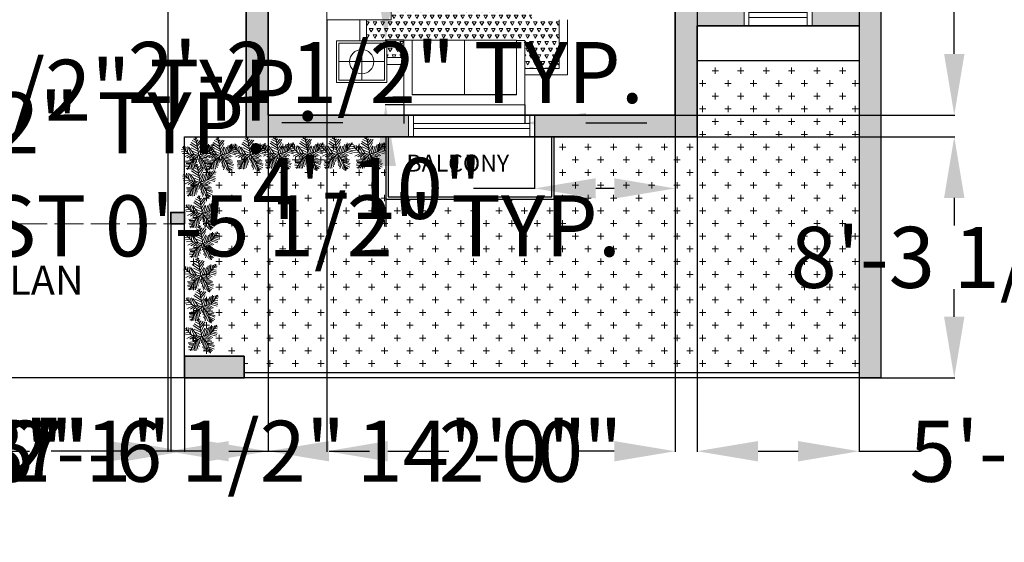
# Model space of a CAD drawing. Units: inches. Extents: x 29 to 6336, y 3 to 2592.
# Tile 4 of 8: x 5531 to 5938, y 1885 to 2100. Entities that reach past the tile are written whole.
import ezdxf

# ---------------------------------------------------------------- set-up
doc = ezdxf.new("R2010")
doc.units = ezdxf.units.IN
doc.header["$MEASUREMENT"] = 0
doc.linetypes.add('ACAD_ISO02W100', pattern=[15, 12, -3])
for name, color, linetype, lineweight in [('A-ANNO-DIMS', 2, 'Continuous', 18), ('A-ANNO-TEXT', 7, 'Continuous', 25), ('A-AREA-IDEN', 7, 'Continuous', 18), ('A-COLS', 7, 'Continuous', 35), ('A-COLS-PATT', 18, 'Continuous', 13), ('A-FLOR', 7, 'Continuous', 25), ('A-FLOR-OVHD', 8, 'ACAD_ISO02W100', 18), ('A-FLOR-PATT', 9, 'Continuous', 13), ('A-FURN', 8, 'Continuous', 18), ('A-GLAZ', 116, 'Continuous', 18), ('A-WALL', 7, 'Continuous', 35), ('A-WALL-PATT', 242, 'Continuous', 13), ('C-PROP', 7, 'Continuous', 25), ('L-PLNT', 94, 'Continuous', 18), ('L-PLNT-PATT', 114, 'Continuous', 13)]:
    doc.layers.add(name, color=color, linetype=linetype, lineweight=lineweight)
doc.styles.get("Standard").update_dxf_attribs({"font": 'arial.ttf'})
doc.dimstyles.get("Standard").update_dxf_attribs({"dimtxt": 25.18, "dimasz": 25.18, "dimexe": 0.18, "dimexo": 0.0625, "dimgap": 0.09, "dimtad": 0, "dimtih": 1, "dimtoh": 1, "dimdec": 0, "dimzin": 0, "dimdsep": 46, "dimlunit": 3, "dimtxsty": 'Standard', "dimcen": 0.09, "dimadec": 0, "dimazin": 0, "dimtfac": 1, "dimtdec": 0, "dimtofl": 0, "dimtmove": 0, "dimatfit": 3, "dimfxl": 1, "dimtolj": 1, "dimtzin": 0, "dimarcsym": 0})

# ---------------------------------------------------------------- blocks, each defined once
blk = doc.blocks.new('*U2')
for p, q in [((-3.665, 19.273), (-27.574, 35.527)), ((-5.114, 28.097), (-24.676, 40.636)), ((-7.288, 39.707), (-21.778, 46.673)), ((-8.737, 47.138), (-17.069, 52.711)), ((-10.186, 53.64), (-13.084, 55.962)), ((0, 0), (-10.5, 57)), ((-9.099, 51.782), (-6.563, 55.962)), ((-7.65, 43.423), (-2.578, 49.46)), ((-5.839, 35.992), (4.667, 48.067)), ((-5.114, 27.632), (10.463, 46.673)), ((-2.941, 16.486), (8.652, 37.85)), ((16.259, 5.805), (23.142, 31.348)), ((22.055, 7.198), (27.489, 32.277)), ((27, 9), (48, 36)), ((27.127, 9.056), (31.112, 35.992)), ((35.096, 32.741), (37.27, 22.524)), ((38.719, 34.134), (41.979, 28.561)), ((44.153, 36.456), (45.239, 32.741)), ((-47.498, 19.737), (-55.83, 18.344)), ((-40.615, 13.7), (-55.105, 10.913)), ((-31.5, 4.5), (-52.5, 25.5)), ((-33.37, 6.269), (-52.207, 5.34)), ((-48.585, 21.131), (-49.309, 29.026)), ((-28.299, 3.483), (-47.86, -5.805)), ((-43.513, 28.561), (-42.427, 15.558)), ((-38.442, 26.239), (-34.819, 7.663)), ((-21.416, 3.018), (-38.079, -8.128)), ((-35.544, 28.097), (-24.314, 3.947)), ((0, 0), (-31.5, 4.5)), ((-14.533, 2.09), (-30.834, 25.31)), ((-15.982, 2.09), (-30.11, -9.521)), ((-24.314, 23.917), (-2.941, 13.7)), ((0, 0), (-22.5, -19.5)), ((-6.563, 1.161), (-21.416, -8.128)), ((-20.691, 13.7), (-1.129, 4.876)), ((-1.129, 6.734), (9.014, 26.704)), ((0, 0), (27, 9)), ((0, 0), (18, -22.5)), ((3.942, 1.625), (11.187, 24.381)), ((6.478, 1.625), (26.04, -8.592)), ((10.101, 3.483), (17.708, 26.239)), ((11.187, 3.483), (30.749, -5.805)), ((18.07, 5.805), (35.096, -3.483)), ((24.229, 7.663), (46.688, 1.625)), ((29.662, 12.307), (48.137, 6.269)), ((31.836, 30.883), (32.561, 16.486)), ((33.285, 16.486), (48.862, 10.913)), ((36.183, 19.737), (48.137, 17.88)), ((40.53, 25.775), (48.862, 24.846)), ((43.791, 29.954), (51.036, 30.883)), ((-17.431, -15.094), (-42.789, -18.809)), ((-28.299, -29.026), (-42.789, -31.348)), ((-24.314, -21.596), (-42.427, -22.06)), ((-26.849, -26.24), (-40.253, -25.775)), ((-22.5, -19.5), (-37.5, -45)), ((-15.257, -12.772), (-30.11, -12.772)), ((-29.023, -30.884), (-27.936, -43.887)), ((-25.038, -23.918), (-22.865, -45.281)), ((-20.691, -18.345), (-17.793, -44.352)), ((-6.563, -5.805), (-19.967, -9.985)), ((-17.069, -15.094), (-12.721, -40.172)), ((-13.446, -11.378), (-8.737, -32.741)), ((-9.461, -8.592), (-6.201, -23.453)), ((-4.752, -3.483), (-3.665, -14.629)), ((2.493, -3.019), (-1.491, -20.202)), ((1.769, -2.555), (24.229, -9.521)), ((5.029, -6.27), (2.131, -25.775)), ((9.014, -11.378), (3.58, -35.992)), ((14.085, -16.951), (6.478, -40.172)), ((7.565, -9.056), (32.198, -14.629)), ((18.07, -22.524), (8.289, -45.745)), ((12.274, -15.094), (36.907, -18.809)), ((20.244, -30.419), (15.897, -44.816)), ((16.259, -19.738), (36.183, -22.989)), ((18, -22.5), (27, -52.5)), ((18.433, -22.524), (40.53, -29.026)), ((19.157, -25.311), (38.719, -33.206)), ((-30.834, -34.135), (-42.427, -35.528)), ((-34.457, -39.708), (-40.978, -42.494)), ((-32.646, -36.921), (-31.921, -44.352)), ((22.78, -37.85), (19.519, -48.532)), ((21.331, -32.741), (39.081, -40.636)), ((22.78, -38.314), (34.372, -44.816)), ((24.591, -45.745), (23.142, -50.854)), ((24.591, -43.423), (30.749, -47.603)), ((26.764, -49.925), (28.213, -50.854))]:
    blk.add_line(p, q)
blk = doc.blocks.new('WIN-48')
for p, q in [((0, 9), (0, 0)), ((2, 9), (2, 0)), ((50, 9), (50, 0)), ((52, 9), (52, 0)), ((2, 5.5), (50, 5.5)), ((2, 3.5), (50, 3.5))]:
    blk.add_line(p, q)
blk = doc.blocks.new('WIN-24')
for p, q in [((0, 9), (0, 0)), ((2, 9), (2, 0)), ((26, 9), (26, 0)), ((28, 9), (28, 0)), ((2, 5.5), (26, 5.5)), ((2, 3.5), (26, 3.5))]:
    blk.add_line(p, q)
blk = doc.blocks.new('SOFA-TWO-SEAT')
blk.add_line((4.12, 24.97), (26.62, 24.97))
for points in [[(4.17, 49.94), (0, 49.94), (0, 0), (4.17, 0)], [(4.17, 49.94), (26.62, 49.94), (26.62, 46.51), (4.17, 46.51)], [(4.17, 3.43), (4.17, 46.51)], [(4.12, 3.43), (26.57, 3.43), (26.57, 0), (4.12, 0)]]:
    blk.add_lwpolyline(points)
blk.add_lwpolyline([(26.62, 46.51), (4.12, 46.51), (4.12, 3.43), (26.62, 3.43)], close=True)
blk = doc.blocks.new('END-TABLE-21X17')
for p, q in [((10.41, 16.21), (10.41, 1)), ((1, 8.6), (19.81, 8.6))]:
    blk.add_line(p, q)
for points in [[(0, 17.21), (20.81, 17.21), (20.81, 0), (0, 0)], [(1, 16.21), (19.81, 16.21), (19.81, 1), (1, 1)]]:
    blk.add_lwpolyline(points, close=True)
blk.add_circle((10.41, 8.6), 5)
blk = doc.blocks.new('PORCH-POST')
blk.add_lwpolyline([(5.63, 0), (0, 0), (0, 4.72), (5.63, 4.72)], close=True)
blk = doc.blocks.new('*D28')
at = {"layer": 'A-ANNO-DIMS', "color": 0, "lineweight": -2, "transparency": 16777216}
for p, q in [((5689.81, 2064.89), (5689.81, 2057.28)), ((5739.75, 2064.89), (5739.75, 2057.28)), ((5664.63, 2057.46), (5639.45, 2057.46)), ((5764.93, 2057.46), (5790.11, 2057.46))]:
    blk.add_line(p, q, dxfattribs=at)
at = {"layer": 'A-ANNO-DIMS', "color": 0, "transparency": 16777216}
for points in [[(5664.63, 2061.65), (5664.63, 2053.26), (5689.81, 2057.46)], [(5764.93, 2061.65), (5764.93, 2053.26), (5739.75, 2057.46)]]:
    blk.add_solid(points, dxfattribs=at)
at = {"layer": 'Defpoints', "color": 0, "transparency": 16777216}
for p in [(5689.81, 2064.95), (5739.75, 2064.95), (5689.81, 2057.46)]:
    blk.add_point(p, dxfattribs=at)
at = {"layer": 'A-ANNO-DIMS', "color": 0, "transparency": 16777216, "insert": (5509.91, 2057.46), "char_height": 25.18, "attachment_point": 5}
blk.add_mtext('\\A1;SOFA 4\'-2" TYP.', dxfattribs=at)
blk = doc.blocks.new('*D29')
at = {"layer": 'A-ANNO-DIMS', "color": 0, "lineweight": -2, "transparency": 16777216}
for p, q in [((5682.32, 2116.75), (5682.32, 2141.93)), ((5689.75, 2091.57), (5682.14, 2091.57)), ((5689.75, 2064.95), (5682.14, 2064.95)), ((5682.32, 2039.77), (5682.32, 2014.59))]:
    blk.add_line(p, q, dxfattribs=at)
at = {"layer": 'A-ANNO-DIMS', "color": 0, "transparency": 16777216}
for points in [[(5678.12, 2116.75), (5686.52, 2116.75), (5682.32, 2091.57)], [(5678.12, 2039.77), (5686.52, 2039.77), (5682.32, 2064.95)]]:
    blk.add_solid(points, dxfattribs=at)
at = {"layer": 'Defpoints', "color": 0, "transparency": 16777216}
for p in [(5682.32, 2091.57), (5689.81, 2091.57), (5689.81, 2064.95)]:
    blk.add_point(p, dxfattribs=at)
at = {"layer": 'A-ANNO-DIMS', "color": 0, "transparency": 16777216, "insert": (5682.32, 2078.26), "char_height": 25.18, "attachment_point": 5}
blk.add_mtext('\\A1;2\'-2 1/2" TYP.', dxfattribs=at)
blk = doc.blocks.new('*D34')
at = {"layer": 'A-ANNO-DIMS', "color": 0, "lineweight": -2, "transparency": 16777216}
for p, q in [((5638.44, 2177.3), (5613.26, 2177.3)), ((5663.62, 2174.24), (5663.62, 2177.48)), ((5684.43, 2174.24), (5684.43, 2177.48)), ((5709.61, 2177.3), (5734.79, 2177.3))]:
    blk.add_line(p, q, dxfattribs=at)
at = {"layer": 'A-ANNO-DIMS', "color": 0, "transparency": 16777216}
for points in [[(5638.44, 2181.49), (5638.44, 2173.1), (5663.62, 2177.3)], [(5709.61, 2181.49), (5709.61, 2173.1), (5684.43, 2177.3)]]:
    blk.add_solid(points, dxfattribs=at)
at = {"layer": 'Defpoints', "color": 0, "transparency": 16777216}
for p in [(5663.62, 2174.18), (5684.43, 2177.3), (5684.43, 2174.18)]:
    blk.add_point(p, dxfattribs=at)
at = {"layer": 'A-ANNO-DIMS', "color": 0, "transparency": 16777216, "insert": (5913.59, 2177.3), "char_height": 25.18, "attachment_point": 5}
blk.add_mtext('\\A1;END TABLE 1\'-9" TYP.', dxfattribs=at)
blk = doc.blocks.new('*D38')
at = {"layer": 'A-ANNO-DIMS', "color": 0, "lineweight": -2, "transparency": 16777216}
for p, q in [((5410.6, 2015.81), (5410.6, 2014.84)), ((5416.23, 2015.81), (5416.23, 2014.84)), ((5385.42, 2015.02), (5360.24, 2015.02)), ((5441.41, 2015.02), (5466.59, 2015.02))]:
    blk.add_line(p, q, dxfattribs=at)
at = {"layer": 'A-ANNO-DIMS', "color": 0, "transparency": 16777216}
for points in [[(5385.42, 2019.22), (5385.42, 2010.83), (5410.6, 2015.02)], [(5441.41, 2019.22), (5441.41, 2010.83), (5416.23, 2015.02)]]:
    blk.add_solid(points, dxfattribs=at)
at = {"layer": 'Defpoints', "color": 0, "transparency": 16777216}
for p in [(5410.6, 2015.87), (5416.23, 2015.87), (5416.23, 2015.02)]:
    blk.add_point(p, dxfattribs=at)
at = {"layer": 'A-ANNO-DIMS', "color": 0, "transparency": 16777216, "insert": (5624.9, 2015.02), "char_height": 25.18, "attachment_point": 5}
blk.add_mtext('\\A1;POST 0\'-5 1/2" TYP.', dxfattribs=at)
blk = doc.blocks.new('*D39')
at = {"layer": 'A-ANNO-DIMS', "color": 0, "lineweight": -2, "transparency": 16777216}
for p, q in [((5417.07, 2045.77), (5417.07, 2070.95)), ((5417.07, 2070.95), (5442.25, 2070.95)), ((5416.29, 2020.59), (5417.25, 2020.59)), ((5416.29, 2015.87), (5417.25, 2015.87)), ((5417.07, 1990.69), (5417.07, 1965.51))]:
    blk.add_line(p, q, dxfattribs=at)
at = {"layer": 'A-ANNO-DIMS', "color": 0, "transparency": 16777216}
for points in [[(5412.88, 2045.77), (5421.27, 2045.77), (5417.07, 2020.59)], [(5412.88, 1990.69), (5421.27, 1990.69), (5417.07, 2015.87)]]:
    blk.add_solid(points, dxfattribs=at)
at = {"layer": 'Defpoints', "color": 0, "transparency": 16777216}
for p in [(5416.23, 2020.59), (5417.07, 2020.59), (5416.23, 2015.87)]:
    blk.add_point(p, dxfattribs=at)
at = {"layer": 'A-ANNO-DIMS', "color": 0, "transparency": 16777216, "insert": (5548.42, 2070.95), "char_height": 25.18, "attachment_point": 5}
blk.add_mtext('\\A1;0\'-4 1/2" TYP.', dxfattribs=at)
blk = doc.blocks.new('*D49')
at = {"layer": 'A-ANNO-DIMS', "color": 0, "lineweight": -2, "transparency": 16777216}
for p, q in [((5419.6, 2191.59), (5419.6, 1921.9)), ((5510.11, 2191.59), (5510.11, 1921.9)), ((5444.78, 1922.08), (5484.93, 1922.08)), ((5510.11, 1922.08), (5535.29, 1922.08))]:
    blk.add_line(p, q, dxfattribs=at)
at = {"layer": 'A-ANNO-DIMS', "color": 0, "transparency": 16777216}
for points in [[(5444.78, 1926.28), (5444.78, 1917.88), (5419.6, 1922.08)], [(5484.93, 1926.28), (5484.93, 1917.88), (5510.11, 1922.08)]]:
    blk.add_solid(points, dxfattribs=at)
at = {"layer": 'Defpoints', "color": 0, "transparency": 16777216}
for p in [(5419.6, 2191.65), (5510.11, 2191.65), (5510.11, 1922.08)]:
    blk.add_point(p, dxfattribs=at)
at = {"layer": 'A-ANNO-DIMS', "color": 0, "transparency": 16777216, "insert": (5598.08, 1922.08), "char_height": 25.18, "attachment_point": 5}
blk.add_mtext('\\A1;7\'-6 1/2"', dxfattribs=at)
blk = doc.blocks.new('*D52')
at = {"layer": 'A-ANNO-DIMS', "color": 0, "lineweight": -2, "transparency": 16777216}
for p, q in [((5633.77, 2060.65), (5633.77, 1921.9)), ((5801.76, 2060.65), (5801.76, 1921.9)), ((5658.95, 1922.08), (5675.61, 1922.08)), ((5776.58, 1922.08), (5759.92, 1922.08))]:
    blk.add_line(p, q, dxfattribs=at)
at = {"layer": 'A-ANNO-DIMS', "color": 0, "transparency": 16777216}
for points in [[(5658.95, 1926.28), (5658.95, 1917.88), (5633.77, 1922.08)], [(5776.58, 1926.28), (5776.58, 1917.88), (5801.76, 1922.08)]]:
    blk.add_solid(points, dxfattribs=at)
at = {"layer": 'Defpoints', "color": 0, "transparency": 16777216}
for p in [(5633.77, 2060.72), (5801.76, 2060.72), (5801.76, 1922.08)]:
    blk.add_point(p, dxfattribs=at)
at = {"layer": 'A-ANNO-DIMS', "color": 0, "transparency": 16777216, "insert": (5717.77, 1922.08), "char_height": 25.18, "attachment_point": 5}
blk.add_mtext('\\A1;14\'-0"', dxfattribs=at)
blk = doc.blocks.new('*D53')
at = {"layer": 'A-ANNO-DIMS', "color": 0, "lineweight": -2, "transparency": 16777216}
for p, q in [((5801.82, 2182.65), (5917.09, 2182.65)), ((5916.91, 2157.47), (5916.91, 2134.63)), ((5916.91, 2085.9), (5916.91, 2108.74)), ((5801.82, 2060.72), (5917.09, 2060.72))]:
    blk.add_line(p, q, dxfattribs=at)
at = {"layer": 'A-ANNO-DIMS', "color": 0, "transparency": 16777216}
for points in [[(5912.71, 2157.47), (5921.1, 2157.47), (5916.91, 2182.65)], [(5912.71, 2085.9), (5921.1, 2085.9), (5916.91, 2060.72)]]:
    blk.add_solid(points, dxfattribs=at)
at = {"layer": 'Defpoints', "color": 0, "transparency": 16777216}
for p in [(5801.76, 2182.65), (5916.91, 2182.65), (5801.76, 2060.72)]:
    blk.add_point(p, dxfattribs=at)
at = {"layer": 'A-ANNO-DIMS', "color": 0, "transparency": 16777216, "insert": (5916.91, 2121.68), "char_height": 25.18, "attachment_point": 5}
blk.add_mtext('\\A1;10\'-2"', dxfattribs=at)
blk = doc.blocks.new('*D55')
at = {"layer": 'A-ANNO-DIMS', "color": 0, "lineweight": -2, "transparency": 16777216}
for p, q in [((5810.76, 2106.42), (5810.76, 1921.9)), ((5877.66, 2106.42), (5877.66, 1921.9)), ((5835.94, 1922.08), (5852.48, 1922.08)), ((5877.66, 1922.08), (5902.84, 1922.08))]:
    blk.add_line(p, q, dxfattribs=at)
at = {"layer": 'A-ANNO-DIMS', "color": 0, "transparency": 16777216}
for points in [[(5835.94, 1926.28), (5835.94, 1917.88), (5810.76, 1922.08)], [(5852.48, 1926.28), (5852.48, 1917.88), (5877.66, 1922.08)]]:
    blk.add_solid(points, dxfattribs=at)
at = {"layer": 'Defpoints', "color": 0, "transparency": 16777216}
for p in [(5810.76, 2106.48), (5877.66, 2106.48), (5877.66, 1922.08)]:
    blk.add_point(p, dxfattribs=at)
at = {"layer": 'A-ANNO-DIMS', "color": 0, "transparency": 16777216, "insert": (5936.39, 1922.08), "char_height": 25.18, "attachment_point": 5}
blk.add_mtext('\\A1;5\'-7"', dxfattribs=at)
blk = doc.blocks.new('*D56')
at = {"layer": 'A-ANNO-DIMS', "color": 0, "lineweight": -2, "transparency": 16777216}
for p, q in [((5366.79, 1952.27), (5366.79, 1921.9)), ((5599.23, 1952.27), (5599.23, 1921.9)), ((5391.97, 1922.08), (5411.52, 1922.08)), ((5574.05, 1922.08), (5554.5, 1922.08))]:
    blk.add_line(p, q, dxfattribs=at)
at = {"layer": 'A-ANNO-DIMS', "color": 0, "transparency": 16777216}
for points in [[(5391.97, 1926.28), (5391.97, 1917.88), (5366.79, 1922.08)], [(5574.05, 1926.28), (5574.05, 1917.88), (5599.23, 1922.08)]]:
    blk.add_solid(points, dxfattribs=at)
at = {"layer": 'Defpoints', "color": 0, "transparency": 16777216}
for p in [(5366.79, 1952.33), (5599.23, 1952.33), (5599.23, 1922.08)]:
    blk.add_point(p, dxfattribs=at)
at = {"layer": 'A-ANNO-DIMS', "color": 0, "transparency": 16777216, "insert": (5483.01, 1922.08), "char_height": 25.18, "attachment_point": 5}
blk.add_mtext('\\A1;19\'-4 1/2"', dxfattribs=at)
blk = doc.blocks.new('*D57')
at = {"layer": 'A-ANNO-DIMS', "color": 0, "lineweight": -2, "transparency": 16777216}
for p, q in [((5410.6, 2015.81), (5410.6, 1921.9)), ((5593.6, 2015.81), (5593.6, 1921.9)), ((5435.78, 1922.08), (5459.94, 1922.08)), ((5568.42, 1922.08), (5544.25, 1922.08))]:
    blk.add_line(p, q, dxfattribs=at)
at = {"layer": 'A-ANNO-DIMS', "color": 0, "transparency": 16777216}
for points in [[(5435.78, 1926.28), (5435.78, 1917.88), (5410.6, 1922.08)], [(5568.42, 1926.28), (5568.42, 1917.88), (5593.6, 1922.08)]]:
    blk.add_solid(points, dxfattribs=at)
at = {"layer": 'Defpoints', "color": 0, "transparency": 16777216}
for p in [(5410.6, 2015.87), (5593.6, 2015.87), (5593.6, 1922.08)]:
    blk.add_point(p, dxfattribs=at)
at = {"layer": 'A-ANNO-DIMS', "color": 0, "transparency": 16777216, "insert": (5502.1, 1922.08), "char_height": 25.18, "attachment_point": 5}
blk.add_mtext('\\A1;15\'-3"', dxfattribs=at)
blk = doc.blocks.new('*D59')
at = {"layer": 'A-ANNO-DIMS', "color": 0, "lineweight": -2, "transparency": 16777216}
for p, q in [((5519.11, 2182.59), (5519.11, 1921.9)), ((5592.36, 2182.59), (5592.36, 1921.9)), ((5493.93, 1922.08), (5468.75, 1922.08)), ((5617.54, 1922.08), (5642.72, 1922.08))]:
    blk.add_line(p, q, dxfattribs=at)
at = {"layer": 'A-ANNO-DIMS', "color": 0, "transparency": 16777216}
for points in [[(5493.93, 1926.28), (5493.93, 1917.88), (5519.11, 1922.08)], [(5617.54, 1926.28), (5617.54, 1917.88), (5592.36, 1922.08)]]:
    blk.add_solid(points, dxfattribs=at)
at = {"layer": 'Defpoints', "color": 0, "transparency": 16777216}
for p in [(5519.11, 2182.65), (5592.36, 2182.65), (5592.36, 1922.08)]:
    blk.add_point(p, dxfattribs=at)
at = {"layer": 'A-ANNO-DIMS', "color": 0, "transparency": 16777216, "insert": (5555.73, 1922.08), "char_height": 25.18, "attachment_point": 5}
blk.add_mtext('\\A1;6\'-1"', dxfattribs=at)
blk = doc.blocks.new('*D61')
at = {"layer": 'A-ANNO-DIMS', "color": 0, "lineweight": -2, "transparency": 16777216}
for p, q in [((5810.82, 2051.72), (5917.09, 2051.72)), ((5916.91, 2026.54), (5916.91, 2015.14)), ((5916.91, 1977.51), (5916.91, 1988.91)), ((5877.72, 1952.33), (5917.09, 1952.33))]:
    blk.add_line(p, q, dxfattribs=at)
at = {"layer": 'A-ANNO-DIMS', "color": 0, "transparency": 16777216}
for points in [[(5912.71, 2026.54), (5921.1, 2026.54), (5916.91, 2051.72)], [(5912.71, 1977.51), (5921.1, 1977.51), (5916.91, 1952.33)]]:
    blk.add_solid(points, dxfattribs=at)
at = {"layer": 'Defpoints', "color": 0, "transparency": 16777216}
for p in [(5810.76, 2051.72), (5877.66, 1952.33), (5916.91, 1952.33)]:
    blk.add_point(p, dxfattribs=at)
at = {"layer": 'A-ANNO-DIMS', "color": 0, "transparency": 16777216, "insert": (5916.91, 2002.02), "char_height": 25.18, "attachment_point": 5}
blk.add_mtext('\\A1;8\'-3 1/2"', dxfattribs=at)
blk = doc.blocks.new('*D64')
at = {"layer": 'A-ANNO-DIMS', "color": 0, "lineweight": -2, "transparency": 16777216}
for p, q in [((5743.77, 2060.65), (5743.77, 2030.29)), ((5801.76, 2060.65), (5801.76, 2030.29)), ((5743.77, 2030.47), (5718.59, 2030.47)), ((5776.58, 2030.47), (5768.95, 2030.47))]:
    blk.add_line(p, q, dxfattribs=at)
at = {"layer": 'A-ANNO-DIMS', "color": 0, "transparency": 16777216}
for points in [[(5768.95, 2034.66), (5768.95, 2026.27), (5743.77, 2030.47)], [(5776.58, 2034.66), (5776.58, 2026.27), (5801.76, 2030.47)]]:
    blk.add_solid(points, dxfattribs=at)
at = {"layer": 'Defpoints', "color": 0, "transparency": 16777216}
for p in [(5743.77, 2060.72), (5801.76, 2060.72), (5743.77, 2030.47)]:
    blk.add_point(p, dxfattribs=at)
at = {"layer": 'A-ANNO-DIMS', "color": 0, "transparency": 16777216, "insert": (5674.74, 2030.47), "char_height": 25.18, "attachment_point": 5}
blk.add_mtext('\\A1;4\'-10"', dxfattribs=at)
blk = doc.blocks.new('*D66')
at = {"layer": 'A-ANNO-DIMS', "color": 0, "lineweight": -2, "transparency": 16777216}
for p, q in [((5658, 2099.97), (5658, 1921.9)), ((5633.77, 2060.65), (5633.77, 1921.9)), ((5608.59, 1922.08), (5583.41, 1922.08)), ((5683.18, 1922.08), (5708.36, 1922.08))]:
    blk.add_line(p, q, dxfattribs=at)
at = {"layer": 'A-ANNO-DIMS', "color": 0, "transparency": 16777216}
for points in [[(5608.59, 1926.28), (5608.59, 1917.88), (5633.77, 1922.08)], [(5683.18, 1926.28), (5683.18, 1917.88), (5658, 1922.08)]]:
    blk.add_solid(points, dxfattribs=at)
at = {"layer": 'Defpoints', "color": 0, "transparency": 16777216}
for p in [(5658, 2100.03), (5633.77, 2060.72), (5658, 1922.08)]:
    blk.add_point(p, dxfattribs=at)
at = {"layer": 'A-ANNO-DIMS', "color": 0, "transparency": 16777216, "insert": (5742.14, 1922.08), "char_height": 25.18, "attachment_point": 5}
blk.add_mtext('\\A1;2\'-0"', dxfattribs=at)

msp = doc.modelspace()

# ---------------------------------------------------------------- hatches: boundary and pattern name
at = {"layer": 'A-COLS-PATT'}
h = msp.add_hatch(color=256, dxfattribs=at)
h.dxf.hatch_style = 1
h.paths.add_polyline_path([(5416.23, 2020.59), (5410.6, 2020.59), (5410.6, 2015.87), (5416.23, 2015.87)])
h.paths.add_polyline_path([(5599.23, 2020.59), (5593.6, 2020.59), (5593.6, 2015.87), (5599.23, 2015.87)])
h = msp.add_hatch(color=256, dxfattribs=at)
h.dxf.hatch_style = 1
h.paths.add_polyline_path([(5623.93, 1961.33), (5599.23, 1961.33), (5599.23, 1952.33), (5623.93, 1952.33)])
at = {"layer": 'A-FLOR-PATT'}
h = msp.add_hatch(dxfattribs=at)
h.set_pattern_fill('TRIANG', color=256, scale=8.4)
h.paths.add_polyline_path([(5742.55, 2146.54), (5742.55, 2149.97), (5754.06, 2149.97), (5754.06, 2166.16), (5684.43, 2166.16), (5684.43, 2156.97), (5674.45, 2156.97), (5674.45, 2149.97), (5684.63, 2149.97), (5684.63, 2146.54), (5684.63, 2103.46), (5684.58, 2103.46), (5684.58, 2100.03), (5674.45, 2100.03), (5674.45, 2091.34), (5682.83, 2091.34), (5682.83, 2084.5), (5689.81, 2084.5), (5689.81, 2091.57), (5693.24, 2091.57), (5736.32, 2091.57), (5736.32, 2091.52), (5739.75, 2091.52), (5739.75, 2079.85), (5753.82, 2079.85), (5753.82, 2100.03), (5742.6, 2100.03), (5742.6, 2103.46), (5742.55, 2103.46)])
h.paths.add_polyline_path([(5722.48, 2132.65), (5722.48, 2113.77), (5704, 2113.77), (5704, 2132.65)], flags=16)
at = {"layer": 'A-WALL-PATT'}
h = msp.add_hatch(color=256, dxfattribs=at)
h.dxf.hatch_style = 1
h.paths.add_polyline_path([(5558.68, 2492.33), (5459.71, 2492.33), (5459.71, 2483.33), (5511.77, 2483.33), (5511.77, 2388.68), (5520.77, 2388.68), (5520.77, 2393.05), (5526.31, 2393.05), (5526.31, 2402.05), (5520.77, 2402.05), (5520.77, 2483.33), (5558.68, 2483.33)])
h.paths.add_polyline_path([(5659.13, 2492.33), (5586.68, 2492.33), (5586.68, 2483.33), (5624.6, 2483.33), (5624.6, 2402.05), (5562.29, 2402.05), (5562.29, 2393.05), (5676.48, 2393.05), (5676.48, 2402.05), (5633.6, 2402.05), (5633.6, 2422.71), (5633.6, 2483.33), (5659.13, 2483.33)])
h.paths.add_polyline_path([(5886.66, 2492.33), (5687.13, 2492.33), (5687.13, 2483.33), (5712.66, 2483.33), (5712.66, 2468.69), (5721.66, 2468.69), (5721.66, 2483.33), (5877.66, 2483.33), (5877.66, 2106.48), (5858.21, 2106.48), (5858.21, 2097.48), (5877.66, 2097.48), (5877.66, 1961.33), (5877.66, 1952.33), (5886.66, 1952.33)])
h.paths.add_polyline_path([(5721.66, 2416.69), (5712.66, 2416.69), (5712.66, 2402.05), (5709.45, 2402.05), (5709.45, 2393.05), (5712.66, 2393.05), (5712.66, 2386.01), (5721.66, 2386.01)], flags=17)
h.paths.add_polyline_path([(5355.66, 2483.33), (5407.71, 2483.33), (5407.71, 2492.33), (5346.66, 2492.33), (5346.66, 2431.95), (5355.66, 2431.95)])
h.paths.add_polyline_path([(5355.66, 2379.95), (5346.66, 2379.95), (5346.66, 2319.56), (5355.66, 2319.56), (5355.66, 2328.56)])
h.paths.add_polyline_path([(5520.77, 2337.13), (5511.77, 2337.13), (5511.77, 2328.56), (5410.6, 2328.56), (5410.6, 2319.56), (5410.6, 2281.61), (5419.6, 2281.61), (5419.6, 2319.56), (5510.11, 2319.56), (5510.11, 2234.67), (5519.11, 2234.67), (5519.11, 2319.56), (5520.77, 2319.56)])
h.paths.add_polyline_path([(5519.11, 2197.33), (5510.11, 2197.33), (5510.11, 2191.65), (5419.6, 2191.65), (5419.6, 2228.6), (5419.6, 2229.61), (5410.6, 2229.61), (5410.6, 2182.65), (5519.11, 2182.65)])
h.paths.add_polyline_path([(5712.66, 2193.6), (5592.36, 2193.6), (5592.36, 2182.65), (5624.77, 2182.65), (5633.77, 2182.65), (5712.66, 2182.65)])
h.paths.add_polyline_path([(5633.77, 2182.65), (5624.77, 2182.65), (5624.77, 2051.72), (5633.77, 2051.72), (5691.77, 2051.72), (5691.77, 2060.72), (5633.77, 2060.72)])
h.paths.add_polyline_path([(5810.76, 2097.48), (5830.21, 2097.48), (5830.21, 2106.48), (5810.76, 2106.48), (5810.76, 2182.65), (5817.87, 2182.65), (5817.87, 2193.6), (5783.59, 2193.6), (5783.59, 2182.65), (5801.76, 2182.65), (5801.76, 2060.72), (5743.77, 2060.72), (5743.77, 2051.72), (5810.76, 2051.72)], flags=17)
h.paths.add_polyline_path([(5721.66, 2319.56), (5877.66, 2319.56), (5877.66, 2328.56), (5721.66, 2328.56), (5721.66, 2335.85), (5712.66, 2335.85), (5712.66, 2319.56), (5712.66, 2182.65), (5726.12, 2182.65), (5726.12, 2193.6), (5721.66, 2193.6)], flags=17)
h.paths.add_polyline_path([(5631.73, 2431.78), (5711.31, 2431.78), (5711.31, 2446.2), (5631.73, 2446.2)], flags=9)
at = {"layer": 'L-PLNT-PATT'}
h = msp.add_hatch(dxfattribs=at)
h.set_pattern_fill('CROSS', color=256, scale=21)
h.paths.add_polyline_path([(5877.66, 2083.16), (5810.76, 2083.16), (5810.76, 2051.72), (5751.88, 2051.72), (5751.88, 2026.05), (5682.34, 2026.05), (5682.34, 2051.72), (5633.77, 2051.72), (5599.23, 2051.72), (5599.23, 1961.33), (5623.93, 1961.33), (5623.93, 1954.59), (5877.66, 1954.59)])
h.paths.add_polyline_path([(5678.67, 2039.6), (5678.66, 2039.59), (5678.67, 2039.58)], flags=16)
h.paths.add_polyline_path([(5677.53, 2042.29), (5677.45, 2042.05), (5677.76, 2042)], flags=16)
h.paths.add_polyline_path([(5671.69, 2040.12), (5671.46, 2040.09), (5671.49, 2039.78)], flags=16)
h.paths.add_polyline_path([(5673, 2042.52), (5673.04, 2042.22), (5673.47, 2042.59)], flags=16)
h.paths.add_polyline_path([(5665.32, 2039.6), (5665.32, 2039.59), (5665.33, 2039.58)], flags=16)
h.paths.add_polyline_path([(5664.19, 2042.29), (5664.11, 2042.05), (5664.42, 2042)], flags=16)
h.paths.add_polyline_path([(5658.35, 2040.12), (5658.12, 2040.09), (5658.15, 2039.78)], flags=16)
h.paths.add_polyline_path([(5659.66, 2042.52), (5659.69, 2042.22), (5660.12, 2042.59)], flags=16)
h.paths.add_polyline_path([(5653.28, 2039.6), (5653.28, 2039.59), (5653.29, 2039.58)], flags=16)
h.paths.add_polyline_path([(5652.15, 2042.29), (5652.07, 2042.05), (5652.38, 2042)], flags=16)
h.paths.add_polyline_path([(5646.31, 2040.12), (5646.08, 2040.09), (5646.11, 2039.78)], flags=16)
h.paths.add_polyline_path([(5647.62, 2042.52), (5647.65, 2042.22), (5648.08, 2042.59)], flags=16)
h.paths.add_polyline_path([(5641.1, 2039.6), (5641.09, 2039.59), (5641.1, 2039.58)], flags=16)
h.paths.add_polyline_path([(5639.96, 2042.29), (5639.88, 2042.05), (5640.19, 2042)], flags=16)
h.paths.add_polyline_path([(5634.12, 2040.12), (5633.89, 2040.09), (5633.92, 2039.78)], flags=16)
h.paths.add_polyline_path([(5635.43, 2042.52), (5635.47, 2042.22), (5635.9, 2042.59)], flags=16)
h.paths.add_polyline_path([(5629.49, 2039.31), (5629.49, 2039.3), (5629.5, 2039.29)], flags=16)
h.paths.add_polyline_path([(5628.36, 2042), (5628.28, 2041.76), (5628.59, 2041.71)], flags=16)
h.paths.add_polyline_path([(5622.52, 2039.83), (5622.29, 2039.8), (5622.32, 2039.49)], flags=16)
h.paths.add_polyline_path([(5623.83, 2042.23), (5623.86, 2041.93), (5624.29, 2042.3)], flags=16)
h.paths.add_polyline_path([(5617.31, 2039.17), (5617.3, 2039.15), (5617.31, 2039.15)], flags=16)
h.paths.add_polyline_path([(5616.17, 2041.85), (5616.09, 2041.61), (5616.4, 2041.56)], flags=16)
h.paths.add_polyline_path([(5611.32, 2036.97), (5611.67, 2037.02), (5611.59, 2037.32)], flags=16)
h.paths.add_polyline_path([(5609.19, 2034), (5609.23, 2034.27), (5608.77, 2034.12)], flags=16)
h.paths.add_polyline_path([(5608.17, 2039.17), (5608.16, 2039.15), (5608.17, 2039.15)], flags=16)
h.paths.add_polyline_path([(5605.32, 2035.22), (5605.45, 2035.45), (5605.26, 2035.59)], flags=16)
h.paths.add_polyline_path([(5601.19, 2039.68), (5600.96, 2039.65), (5600.99, 2039.34)], flags=16)
h.paths.add_polyline_path([(5603.32, 2042.45), (5602.96, 2042.45), (5603.01, 2042.19)], flags=16)
h.paths.add_polyline_path([(5607.03, 2041.85), (5606.95, 2041.61), (5607.26, 2041.56)], flags=16)
h.paths.add_polyline_path([(5611.29, 2041.31), (5611.09, 2041.31), (5611.12, 2041.02)], flags=16)
h.paths.add_polyline_path([(5611.64, 2042.09), (5611.68, 2041.78), (5612.11, 2042.15)], flags=16)
h.paths.add_polyline_path([(5603.35, 2044.38), (5603.27, 2044.48), (5603.18, 2044.4)], flags=16)
h.paths.add_polyline_path([(5604, 2050.75), (5604.1, 2050.91), (5603.95, 2051.02)], flags=16)
h.paths.add_polyline_path([(5608.41, 2046.56), (5608.45, 2046.71), (5608.29, 2046.68)], flags=16)
h.paths.add_polyline_path([(5608.89, 2045.84), (5608.87, 2046.12), (5608.82, 2045.83)], flags=16)
h.paths.add_polyline_path([(5613.14, 2050.75), (5613.24, 2050.91), (5613.09, 2051.02)], flags=16)
h.paths.add_polyline_path([(5620.14, 2048.2), (5620.16, 2048.01), (5620.32, 2048.03), (5620.24, 2048.33)], flags=16)
h.paths.add_polyline_path([(5624.67, 2044.52), (5624.6, 2044.62), (5624.51, 2044.55)], flags=16)
h.paths.add_polyline_path([(5625.33, 2050.89), (5625.42, 2051.05), (5625.28, 2051.17)], flags=16)
h.paths.add_polyline_path([(5636.27, 2044.81), (5636.2, 2044.91), (5636.11, 2044.84)], flags=16)
h.paths.add_polyline_path([(5643.92, 2048.62), (5643.94, 2048.44), (5644.11, 2048.46), (5644.03, 2048.76)], flags=16)
h.paths.add_polyline_path([(5648.46, 2044.81), (5648.39, 2044.91), (5648.29, 2044.84)], flags=16)
h.paths.add_polyline_path([(5655.98, 2048.46), (5655.98, 2048.42), (5656.3, 2048.46), (5656.21, 2048.76)], flags=16)
h.paths.add_polyline_path([(5660.5, 2044.81), (5660.43, 2044.91), (5660.33, 2044.84)], flags=16)
h.paths.add_polyline_path([(5668.34, 2048.46), (5668.25, 2048.76), (5667.98, 2048.42)], flags=16)
h.paths.add_polyline_path([(5673.84, 2044.81), (5673.77, 2044.91), (5673.68, 2044.84)], flags=16)
h.paths.add_polyline_path([(5681.68, 2048.46), (5681.6, 2048.76), (5681.33, 2048.42)], flags=16)
h.paths.add_polyline_path([(5679.2, 2045.45), (5679.24, 2045.72), (5678.78, 2045.56)], flags=16)
h.paths.add_polyline_path([(5671.41, 2045.36), (5668.98, 2045.24), (5665.97, 2046.22), (5665.86, 2045.45), (5665.43, 2045.56), (5662.88, 2044.71), (5662.94, 2044.9), (5663.14, 2044.8), (5663.68, 2044.98), (5663.71, 2045.05), (5663.79, 2045.01), (5664.47, 2045.24), (5664.52, 2045.41), (5664.69, 2045.31), (5665.24, 2045.5), (5665.27, 2045.61), (5665.43, 2045.56), (5665.9, 2045.72), (5665.97, 2046.22), (5668.98, 2045.24), (5671.25, 2045.35), (5671.21, 2045.56), (5670.45, 2046.32), (5670.25, 2046.28), (5670.23, 2046.54), (5669.65, 2047.12), (5669.45, 2047.08), (5669.42, 2047.35)], flags=16)
h.paths.add_polyline_path([(5658.07, 2045.36), (5656.77, 2045.29), (5653.93, 2046.22), (5653.82, 2045.45), (5653.39, 2045.56), (5650.84, 2044.71), (5650.9, 2044.9), (5651.1, 2044.8), (5651.64, 2044.98), (5651.67, 2045.05), (5651.75, 2045.01), (5652.43, 2045.24), (5652.48, 2045.41), (5652.65, 2045.31), (5653.2, 2045.5), (5653.23, 2045.61), (5653.39, 2045.56), (5653.86, 2045.72), (5653.93, 2046.22), (5654.92, 2045.9), (5656.9, 2046.28), (5656.88, 2046.54), (5656.56, 2046.86), (5655.65, 2047.01), (5656.31, 2047.12), (5655.53, 2047.89), (5656.78, 2047.75), (5656.88, 2046.54)], flags=16)
h.paths.add_polyline_path([(5646.03, 2045.36), (5644.61, 2045.29), (5641.75, 2046.22), (5641.63, 2045.45), (5641.21, 2045.56), (5638.65, 2044.71), (5638.71, 2044.9), (5638.91, 2044.8), (5639.46, 2044.98), (5639.48, 2045.05), (5639.57, 2045.01), (5640.25, 2045.24), (5640.29, 2045.41), (5640.47, 2045.31), (5641.02, 2045.5), (5641.04, 2045.61), (5641.21, 2045.56), (5641.67, 2045.72), (5641.75, 2046.22), (5644.61, 2045.29), (5645.86, 2045.35), (5645.82, 2045.56), (5645.07, 2046.32), (5644.86, 2046.28), (5644.84, 2046.54), (5644.55, 2046.84), (5643.54, 2046.99), (5644.27, 2047.12), (5643.51, 2047.87), (5644.74, 2047.74), (5644.84, 2046.54)], flags=16)
h.paths.add_polyline_path([(5633.11, 2048.25), (5633.64, 2045.56), (5633.84, 2045.36), (5632.16, 2045.27), (5630.39, 2045.85), (5630.07, 2045.45), (5630.03, 2045.16), (5629.6, 2045.27), (5627.05, 2044.42), (5627.11, 2044.61), (5627.31, 2044.51), (5627.85, 2044.69), (5627.88, 2044.76), (5627.96, 2044.72), (5628.64, 2044.95), (5628.69, 2045.12), (5628.86, 2045.02), (5629.41, 2045.21), (5629.44, 2045.32), (5629.6, 2045.27), (5630.05, 2045.42), (5630.07, 2045.45), (5630.14, 2045.93), (5630.39, 2045.85), (5630.77, 2046.35), (5630.75, 2046.89), (5631.26, 2046.98), (5631.39, 2047.14), (5631.21, 2047.99), (5631.58, 2047.62), (5631.75, 2047.6), (5631.82, 2047.7), (5631.76, 2048.35), (5631.91, 2048.1), (5632.16, 2048.13), (5632.49, 2048.56), (5632.52, 2048.17)], flags=16)
h.paths.add_polyline_path([(5622.24, 2045.07), (5620.43, 2044.98), (5617.96, 2045.79), (5617.84, 2045.01), (5617.42, 2045.13), (5614.37, 2044.11), (5611.6, 2044.5), (5610.08, 2043.49), (5609.32, 2043.91), (5608.03, 2043.29), (5605.99, 2044.36), (5605.72, 2044.27), (5605.79, 2044.47), (5605.99, 2044.36), (5606.53, 2044.54), (5606.56, 2044.62), (5606.64, 2044.58), (5607.32, 2044.81), (5607.36, 2044.97), (5607.54, 2044.88), (5608.73, 2045.28), (5609.45, 2046.21), (5609.38, 2047.51), (5609.54, 2046.73), (5609.82, 2046.68), (5610.06, 2047), (5610.03, 2047.18), (5610.09, 2047.03), (5610.37, 2047.39), (5610.31, 2047.47), (5610.42, 2047.46), (5610.68, 2047.79), (5610.59, 2047.95), (5610.83, 2047.98), (5611.1, 2048.33), (5611.03, 2048.55), (5611.7, 2048.09), (5610.83, 2047.98), (5610.37, 2047.39), (5612.48, 2044.38), (5614.37, 2044.11), (5614.86, 2044.27), (5614.92, 2044.47), (5615.12, 2044.36), (5615.67, 2044.54), (5615.69, 2044.62), (5615.78, 2044.58), (5616.46, 2044.81), (5616.5, 2044.97), (5616.68, 2044.88), (5617.23, 2045.06), (5617.25, 2045.17), (5617.42, 2045.13), (5617.88, 2045.28), (5617.96, 2045.79), (5620.43, 2044.98), (5622.07, 2045.06), (5622.03, 2045.27), (5621.28, 2046.03), (5621.08, 2045.99), (5621.05, 2046.25), (5620.93, 2046.38), (5619.3, 2046.63), (5620.48, 2046.83), (5619.89, 2047.42), (5620.97, 2047.3), (5621.05, 2046.25)], flags=16)
h.paths.add_polyline_path([(5609.7, 1976.79), (5609.7, 1976.77), (5609.71, 1976.77)], flags=16)
h.paths.add_polyline_path([(5608.57, 1979.47), (5608.49, 1979.23), (5608.8, 1979.18)], flags=16)
h.paths.add_polyline_path([(5604.55, 1979.78), (5604.5, 1979.77), (5604.07, 1979.4), (5604.44, 1976.08), (5605.34, 1975.48), (5605.19, 1976.29), (5605.15, 1976.33)], flags=16)
h.paths.add_polyline_path([(5604.88, 1982), (5604.81, 1982.1), (5604.72, 1982.02)], flags=16)
h.paths.add_polyline_path([(5605.54, 1988.37), (5605.63, 1988.53), (5605.49, 1988.64)], flags=16)
h.paths.add_polyline_path([(5612.72, 1985.65), (5612.63, 1985.95), (5612.37, 1985.6)], flags=16)
h.paths.add_polyline_path([(5609.04, 1989.51), (5609.04, 1989.5), (5609.05, 1989.49)], flags=16)
h.paths.add_polyline_path([(5607.91, 1992.2), (5607.83, 1991.96), (5608.14, 1991.91)], flags=16)
h.paths.add_polyline_path([(5602.07, 1990.03), (5601.84, 1990), (5601.87, 1989.69)], flags=16)
h.paths.add_polyline_path([(5603.38, 1992.43), (5603.42, 1992.13), (5603.85, 1992.5)], flags=16)
h.paths.add_polyline_path([(5604.22, 1994.72), (5604.15, 1994.82), (5604.06, 1994.75)], flags=16)
h.paths.add_polyline_path([(5604.88, 2001.09), (5604.98, 2001.25), (5604.83, 2001.37)], flags=16)
h.paths.add_polyline_path([(5612.06, 1998.37), (5611.97, 1998.67), (5611.71, 1998.33)], flags=16)
h.paths.add_polyline_path([(5609.81, 2002.86), (5609.81, 2002.84), (5609.82, 2002.84)], flags=16)
h.paths.add_polyline_path([(5608.68, 2005.54), (5608.6, 2005.3), (5608.91, 2005.25)], flags=16)
h.paths.add_polyline_path([(5602.84, 2003.37), (5602.61, 2003.34), (5602.64, 2003.03)], flags=16)
h.paths.add_polyline_path([(5604.15, 2005.78), (5604.18, 2005.47), (5604.61, 2005.85)], flags=16)
h.paths.add_polyline_path([(5604.99, 2008.07), (5604.92, 2008.17), (5604.83, 2008.09)], flags=16)
h.paths.add_polyline_path([(5602.64, 2015.65), (5602.41, 2015.62), (5602.44, 2015.31)], flags=16)
h.paths.add_polyline_path([(5603.95, 2018.05), (5603.98, 2017.75), (5604.41, 2018.12)], flags=16)
h.paths.add_polyline_path([(5605.65, 2014.44), (5605.74, 2014.6), (5605.6, 2014.72)], flags=16)
h.paths.add_polyline_path([(5612.83, 2011.72), (5612.74, 2012.02), (5612.48, 2011.67)], flags=16)
h.paths.add_polyline_path([(5610.35, 2008.7), (5610.39, 2008.97), (5609.92, 2008.82)], flags=16)
h.paths.add_polyline_path([(5610.24, 1982.63), (5610.28, 1982.9), (5609.81, 1982.75)], flags=16)
h.paths.add_polyline_path([(5609.58, 1995.36), (5609.62, 1995.63), (5609.15, 1995.47)], flags=16)
h.paths.add_polyline_path([(5609.4, 1964.43), (5609.4, 1964.42), (5609.41, 1964.41)], flags=16)
h.paths.add_polyline_path([(5608.27, 1967.12), (5608.19, 1966.88), (5608.5, 1966.83)], flags=16)
h.paths.add_polyline_path([(5602.43, 1964.95), (5602.2, 1964.92), (5602.23, 1964.61)], flags=16)
h.paths.add_polyline_path([(5603.74, 1967.35), (5603.78, 1967.05), (5604.21, 1967.42)], flags=16)
h.paths.add_polyline_path([(5604.58, 1969.65), (5604.51, 1969.75), (5604.42, 1969.67)], flags=16)
h.paths.add_polyline_path([(5612.42, 1973.3), (5612.34, 1973.59), (5612.07, 1973.25)], flags=16)
h.paths.add_polyline_path([(5609.61, 2015.13), (5609.61, 2015.12), (5609.62, 2015.11)], flags=16)
h.paths.add_polyline_path([(5608.48, 2017.82), (5608.4, 2017.58), (5608.71, 2017.53)], flags=16)
h.paths.add_polyline_path([(5604.79, 2020.34), (5604.72, 2020.44), (5604.63, 2020.37)], flags=16)
h.paths.add_polyline_path([(5605.45, 2026.71), (5605.54, 2026.87), (5605.4, 2026.99)], flags=16)
h.paths.add_polyline_path([(5612.63, 2023.99), (5612.54, 2024.29), (5612.28, 2023.95)], flags=16)
h.paths.add_polyline_path([(5610.15, 2020.98), (5610.19, 2021.25), (5609.72, 2021.09)], flags=16)
h.paths.add_polyline_path([(5609.94, 1970.28), (5609.98, 1970.55), (5609.52, 1970.39)], flags=16)
h.paths.add_polyline_path([(5608.66, 2028.16), (5608.65, 2028.14), (5608.66, 2028.14)], flags=16)
h.paths.add_polyline_path([(5607.52, 2030.84), (5607.44, 2030.6), (5607.75, 2030.55)], flags=16)
h.paths.add_polyline_path([(5610.64, 2039.72), (5610.1, 2039.65), (5610.18, 2038.89), (5608.82, 2039.5), (5610.5, 2039.7), (5607.46, 2040.93), (5607.57, 2041.2), (5610.56, 2040.32), (5610.59, 2040.33)], flags=16)
h.paths.add_polyline_path([(5602.73, 1977.3), (5602.5, 1977.27), (5602.53, 1976.96)], flags=16)
h.paths.add_polyline_path([(5602.56, 2008.61), (5602.39, 2008.61), (5602.35, 2008.82), (5601.6, 2009.57), (5601.4, 2009.54), (5601.37, 2009.8), (5600.8, 2010.37), (5600.59, 2010.34), (5600.57, 2010.6)], flags=16)
h.paths.add_polyline_path([(5602.45, 1982.54), (5602.29, 1982.53), (5602.24, 1982.75), (5601.49, 1983.5), (5601.29, 1983.46), (5601.26, 1983.73), (5600.69, 1984.3), (5600.48, 1984.27), (5600.46, 1984.53)], flags=16)
h.paths.add_polyline_path([(5601.79, 1995.27), (5601.63, 1995.26), (5601.58, 1995.47)], flags=16)
h.paths.add_polyline_path([(5601.68, 2028.67), (5601.45, 2028.64), (5601.48, 2028.33)], flags=16)
h.paths.add_polyline_path([(5602.99, 2031.08), (5603.03, 2030.77), (5603.46, 2031.14)], flags=16)
h.paths.add_polyline_path([(5603.83, 2033.37), (5603.76, 2033.47), (5603.67, 2033.39)], flags=16)
h.paths.add_polyline_path([(5602.36, 2020.89), (5602.19, 2020.88), (5602.15, 2021.09), (5601.4, 2021.85), (5601.2, 2021.81), (5601.17, 2022.07), (5600.6, 2022.65), (5600.39, 2022.61), (5600.37, 2022.88)], flags=16)
h.paths.add_polyline_path([(5602.15, 1970.19), (5601.99, 1970.18), (5601.95, 1970.4), (5601.19, 1971.15), (5600.99, 1971.11), (5600.97, 1971.38)], flags=16)

# ---------------------------------------------------------------- linework, layer by layer
at = {"layer": 'A-COLS'}
msp.add_lwpolyline([(5623.93, 1961.33), (5599.23, 1961.33), (5599.23, 1952.33), (5623.93, 1952.33)], close=True, dxfattribs=at)
at = {"layer": 'A-FLOR'}
for p, q in [((5682.34, 2051.72), (5682.34, 2026.05)), ((5683.34, 2051.72), (5683.34, 2027.05)), ((5750.88, 2027.05), (5750.88, 2051.72)), ((5751.88, 2026.05), (5751.88, 2051.72)), ((5682.34, 2026.05), (5751.88, 2026.05)), ((5683.34, 2027.05), (5750.88, 2027.05))]:
    msp.add_line(p, q, dxfattribs=at)
at = {"layer": 'A-FLOR-OVHD'}
msp.add_line((5410.6, 2015.87), (5599.23, 2015.87), dxfattribs=at)
at = {"layer": 'A-FLOR-PATT'}
for p, q in [((5671.67, 2100.03), (5671.67, 2091.34)), ((5674.45, 2091.34), (5674.45, 2100.03)), ((5753.82, 2100.03), (5753.82, 2079.85)), ((5757.26, 2100.03), (5757.26, 2077.34)), ((5682.83, 2084.5), (5689.81, 2084.5)), ((5682.83, 2081.5), (5689.81, 2081.5)), ((5753.82, 2079.85), (5739.75, 2079.85)), ((5757.26, 2077.34), (5739.75, 2077.34))]:
    msp.add_line(p, q, dxfattribs=at)
at = {"layer": 'A-WALL'}
for p, q in [((5624.77, 2182.65), (5624.77, 2051.72)), ((5633.77, 2182.65), (5633.77, 2060.72)), ((5801.76, 2182.65), (5801.76, 2060.72)), ((5810.76, 2097.48), (5877.66, 2097.48)), ((5810.76, 2097.48), (5810.76, 2051.72)), ((5633.77, 2060.72), (5801.76, 2060.72)), ((5633.77, 2051.72), (5810.76, 2051.72))]:
    msp.add_line(p, q, dxfattribs=at)
at = {"layer": 'C-PROP'}
for p, q in [((5886.66, 2492.33), (5886.66, 1952.33)), ((5877.66, 2097.48), (5877.66, 1961.33)), ((5810.76, 2083.16), (5877.66, 2083.16)), ((5877.66, 2083.16), (5877.66, 1952.33)), ((5599.23, 1952.33), (5599.23, 2051.72)), ((5599.23, 2051.72), (5633.77, 2051.72)), ((5623.93, 1961.33), (5623.93, 1952.33)), ((5623.93, 1954.59), (5877.66, 1954.59)), ((5886.66, 1952.33), (5346.66, 1952.33))]:
    msp.add_line(p, q, dxfattribs=at)

# ---------------------------------------------------------------- block references
at = {"layer": 'A-COLS'}
msp.add_blockref('PORCH-POST', (5593.6, 2015.87), dxfattribs=at)
at = {"layer": 'A-FURN'}
for name, p in [('SOFA-TWO-SEAT', (5658, 2100.03)), ('END-TABLE-21X17', (5662.01, 2074.13))]:
    msp.add_blockref(name, p, dxfattribs=at)
at = {"layer": 'A-FURN', "rotation": 90.00000000000044}
msp.add_blockref('SOFA-TWO-SEAT', (5739.75, 2064.95), dxfattribs=at)
at = {"layer": 'A-GLAZ'}
for name, p in [('WIN-24', (5830.21, 2097.48)), ('WIN-48', (5691.77, 2051.72))]:
    msp.add_blockref(name, p, dxfattribs=at)
at = {"layer": 'L-PLNT', "xscale": 0.129609211949132, "yscale": 0.129609211949132, "zscale": 0.129609211949132}
for p in [(5626.55, 2044.25), (5638.16, 2044.54), (5650.34, 2044.54), (5662.38, 2044.54), (5675.73, 2044.54), (5605.23, 2044.11), (5614.37, 2044.11), (5605.71, 2033.1), (5606.67, 2020.08), (5606.87, 2007.8), (5606.1, 1994.45), (5606.76, 1981.73), (5606.46, 1969.38)]:
    msp.add_blockref('*U2', p, dxfattribs=at)

# ---------------------------------------------------------------- texts
at = {"layer": 'A-ANNO-TEXT', "insert": (5387.94, 1998.58), "char_height": 12, "attachment_point": 1}
msp.add_mtext_dynamic_manual_height_columns('GROUND FLOOR PLAN', width=221.0762, gutter_width=1, heights=[0], dxfattribs=at)
at = {"layer": 'A-AREA-IDEN', "insert": (5690.85, 2044.39), "char_height": 7, "attachment_point": 1}
msp.add_mtext_dynamic_manual_height_columns('BALCONY', width=54.3344, gutter_width=1, heights=[0], dxfattribs=at)

# ---------------------------------------------------------------- dimensions: what is measured, and where the dimension line sits
at = {"layer": 'A-ANNO-DIMS'}
for base, p1, p2, text, picture, middle in [((5684.43, 2177.3), (5663.62, 2174.18), (5684.43, 2174.18), 'END TABLE <> TYP.', '*D34', (5913.59, 2177.3)), ((5416.23, 2015.02), (5410.6, 2015.87), (5416.23, 2015.87), 'POST <> TYP.', '*D38', (5624.9, 2015.02))]:
    dim = msp.add_linear_dim(base=base, p1=p1, p2=p2, text=text, dimstyle='Standard', override={"dimdec": 1, "dimlfac": 1, "dimrnd": 0, "dimzin": 1, "dimdsep": 46, "dimlunit": 4, "dimfrac": 2}, dxfattribs=at)
    dim.commit()
    dim.dimension.update_dxf_attribs({"geometry": picture, "text_midpoint": middle})
for base, p1, p2, picture, middle in [((5510.11, 1922.08), (5419.6, 2191.65), (5510.11, 2191.65), '*D49', (5598.08, 1922.08)), ((5592.3592, 1922.0797), (5519.1102, 2182.6481), (5592.3592, 2182.6517), '*D59', (5555.7347, 1922.0797)), ((5877.66, 1922.08), (5810.76, 2106.48), (5877.66, 2106.48), '*D55', (5936.39, 1922.08)), ((5658, 1922.08), (5633.77, 2060.72), (5658, 2100.03), '*D66', (5742.14, 1922.08)), ((5801.76, 1922.08), (5633.77, 2060.72), (5801.76, 2060.72), '*D52', (5717.77, 1922.08)), ((5593.6, 1922.08), (5410.6, 2015.87), (5593.6, 2015.87), '*D57', (5502.1, 1922.08)), ((5599.23, 1922.08), (5366.79, 1952.33), (5599.23, 1952.33), '*D56', (5483.01, 1922.08))]:
    dim = msp.add_linear_dim(base=base, p1=p1, p2=p2, dimstyle='Standard', override={"dimdec": 1, "dimlfac": 1, "dimrnd": 0, "dimzin": 1, "dimdsep": 46, "dimlunit": 4, "dimfrac": 2}, dxfattribs=at)
    dim.commit()
    dim.dimension.update_dxf_attribs({"geometry": picture, "text_midpoint": middle})
for base, p1, p2, angle, picture, middle in [((5916.91, 2182.65), (5801.76, 2060.72), (5801.76, 2182.65), 90, '*D53', (5916.91, 2121.68)), ((5743.77, 2030.47), (5801.76, 2060.72), (5743.77, 2060.72), 180, '*D64', (5674.74, 2030.47)), ((5916.91, 1952.33), (5810.76, 2051.72), (5877.66, 1952.33), 90, '*D61', (5916.91, 2002.02))]:
    dim = msp.add_linear_dim(base=base, p1=p1, p2=p2, angle=angle, dimstyle='Standard', override={"dimdec": 1, "dimlfac": 1, "dimrnd": 0, "dimzin": 1, "dimdsep": 46, "dimlunit": 4, "dimfrac": 2}, dxfattribs=at)
    dim.commit()
    dim.dimension.update_dxf_attribs({"geometry": picture, "text_midpoint": middle})
for base, p1, p2, angle, text, picture, middle in [((5682.32, 2091.57), (5689.81, 2064.95), (5689.81, 2091.57), 90, '<> TYP.', '*D29', (5682.32, 2078.26)), ((5417.07, 2020.59), (5416.23, 2015.87), (5416.23, 2020.59), 90, '<> TYP.', '*D39', (5548.42, 2070.95)), ((5689.81, 2057.46), (5739.75, 2064.95), (5689.81, 2064.95), 180, 'SOFA <> TYP.', '*D28', (5509.91, 2057.46))]:
    dim = msp.add_linear_dim(base=base, p1=p1, p2=p2, angle=angle, text=text, dimstyle='Standard', override={"dimdec": 1, "dimlfac": 1, "dimrnd": 0, "dimzin": 1, "dimdsep": 46, "dimlunit": 4, "dimfrac": 2}, dxfattribs=at)
    dim.commit()
    dim.dimension.update_dxf_attribs({"geometry": picture, "text_midpoint": middle})

doc.saveas('drawing.dxf')
